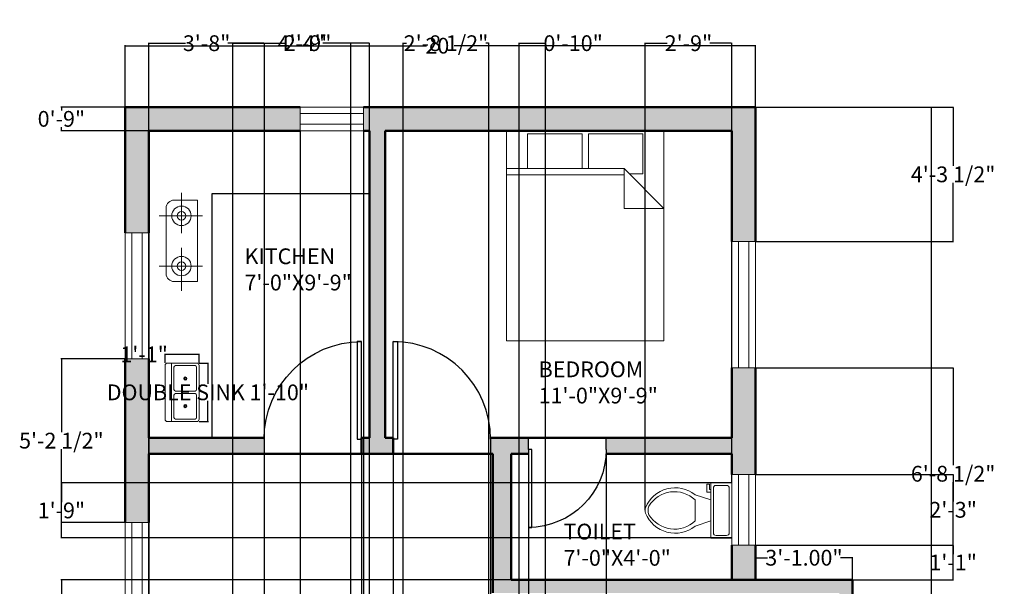
# Model space of a CAD drawing. Units: inches. Extents: x -19 to 356, y -14 to 509.
# Tile 3 of 3: x -19 to 356, y 293 to 509. Entities that reach past the tile are written whole.
import ezdxf

# ---------------------------------------------------------------- set-up
doc = ezdxf.new("R2010")
doc.units = ezdxf.units.IN
doc.header["$MEASUREMENT"] = 0
for name, color, linetype, lineweight in [('A-ANNO-DIMS', 7, 'Continuous', 18), ('A-ANNO-TEXT', 7, 'Continuous', 18), ('A-AREA-IDEN', 7, 'Continuous', 25), ('A-DOOR', 3, 'Continuous', 25), ('A-EQPM', 7, 'Continuous', 18), ('A-FLOR-CASE', 8, 'Continuous', 25), ('A-FLOR-FIXT', 9, 'Continuous', 18), ('A-FURN', 8, 'Continuous', 18), ('A-GLAZ', 5, 'Continuous', 18), ('A-WALL', 7, 'Continuous', 50), ('A-WALL-PATT', 4, 'Continuous', 13)]:
    doc.layers.add(name, color=color, linetype=linetype, lineweight=lineweight)
doc.styles.get("Standard").update_dxf_attribs({"font": 'arial.ttf'})
doc.dimstyles.get("Standard").update_dxf_attribs({"dimtxt": 6, "dimasz": 0.18, "dimexe": 0.18, "dimexo": 0.0625, "dimgap": 0.09, "dimtad": 0, "dimtih": 1, "dimtoh": 1, "dimzin": 0, "dimdsep": 46, "dimlunit": 3, "dimtxsty": 'Standard', "dimcen": 0.09, "dimadec": 0, "dimazin": 0, "dimtfac": 1, "dimtofl": 0, "dimtmove": 0, "dimatfit": 3, "dimfxl": 1, "dimtolj": 1, "dimtzin": 0, "dimarcsym": 0})

# ---------------------------------------------------------------- blocks, each defined once
blk = doc.blocks.new('*U2')
for p, q in [((0, 0), (0, -6)), ((40, 0), (40, -6))]:
    blk.add_line(p, q)
blk.add_lwpolyline([(0, 0), (0, 40), (1.75, 40), (1.75, 0)], close=True)
blk.add_arc((0, 0), 40, 0, 90)
blk = doc.blocks.new('*U4')
for p, q in [((9.5, -6), (9.5, -2)), ((-10, -8.5), (-8, -8.5)), ((-10, -9.5), (-10, -8.5)), ((-7, -9.5), (-10, -9.5)), ((-8, -8.5), (-8, -8)), ((-7, -8), (-7, -9.5)), ((-4, -8), (-6, -14)), ((4, -8), (6, -14)), ((4, -14), (-4, -14))]:
    blk.add_line(p, q)
blk.add_lwpolyline([(10.5, -8), (10.5, 0), (-10.5, 0), (-10.5, -8)], close=True)
for points in [[(-9.5, -2), (-9.5, -6)], [(8.5, -1), (-8.5, -1)], [(-8.5, -7), (8.5, -7)]]:
    blk.add_lwpolyline(points)
for centre, radius, start, end in [((-8.62, -1.88), 0.884, 81.8699, 188.1301), ((8.62, -1.88), 0.884, 351.8699, 98.1301), ((-8.62, -6.12), 0.884, 171.8699, 278.1301), ((8.62, -6.12), 0.884, 261.8699, 8.1301), ((3.52, -21.58), 12.17, 141.4691, 247.9714), ((4.2, -21.82), 11.33, 136.3677, 238.9468), ((-3.52, -21.58), 12.17, 292.0284, 38.5307), ((-4.2, -21.82), 11.33, 301.053, 43.6321), ((0, -27.88), 4, 245.7318, 294.2682), ((0, -29), 4, 254.8605, 285.1395)]:
    blk.add_arc(centre, radius, start, end)
blk = doc.blocks.new('Bed - Queen')
for p, q in [((0, -80.00003), (0, 0)), ((0, 0), (59.99999, 0)), ((59.99999, 0), (59.99999, -80.00003)), ((7.99999, -1.2), (28.79998, -1.2)), ((7.99999, -14.4), (7.99999, -1.2)), ((28.79998, -1.2), (28.79998, -14.4)), ((31.19999, -1.2), (51.99999, -1.2)), ((31.19999, -14.4), (31.19999, -1.2)), ((51.99999, -1.2), (51.99999, -16.4)), ((0, -14.4), (44.8, -14.4)), ((59.99999, -29.6), (44.8, -14.4)), ((44.8, -14.4), (44.8, -29.6)), ((44.8, -16.8), (0, -16.8)), ((51.99999, -16.4), (46.79936, -16.4)), ((44.8, -29.6), (59.99999, -29.6)), ((59.99999, -80.00003), (0, -80.00003))]:
    blk.add_line(p, q)
blk = doc.blocks.new('Sink-double - 36 in top')
for p, q in [((-18, -4), (18, -4)), ((-0.75, -18.5), (-0.75, -6.5)), ((0.75, -6.5), (0.75, -18.5))]:
    blk.add_line(p, q)
for points in [[(-16.5, 0), (16.5, 0)], [(-18, -19.5), (-18, -1.5)], [(-15.5, -5.5), (-1.75, -5.5)], [(1.75, -5.5), (15.5, -5.5)], [(18, -1.5), (18, -19.5)], [(-16.5, -18.5), (-16.5, -6.5)], [(16.5, -6.5), (16.5, -18.5)], [(16.5, -21), (-16.5, -21)], [(-1.75, -19.5), (-15.5, -19.5)], [(15.5, -19.5), (1.75, -19.5)]]:
    blk.add_lwpolyline(points)
for centre, radius in [((-8.5, -12.5), 1), ((-8.5, -12.5), 0.5), ((8.5, -12.5), 1), ((8.5, -12.5), 0.5)]:
    blk.add_circle(centre, radius)
for centre, radius, start, end in [((-16.5, -1.5), 1.5, 90, 180), ((16.5, -1.5), 1.5, 0, 90), ((-15.5, -6.5), 1, 90, 180), ((-1.75, -6.5), 1, 0, 90), ((1.75, -6.5), 1, 90, 180), ((15.5, -6.5), 1, 0, 90), ((-16.5, -19.5), 1.5, 180, 270), ((-15.5, -18.5), 1, 180, 270), ((-1.75, -18.5), 1, 270, 0), ((1.75, -18.5), 1, 180, 270), ((15.5, -18.5), 1, 270, 0), ((16.5, -19.5), 1.5, 270, 0)]:
    blk.add_arc(centre, radius, start, end)
blk = doc.blocks.new('*D7')
at = {"layer": 'A-ANNO-DIMS', "color": 0, "lineweight": -2, "transparency": 16777216}
for p, q in [((21.6, 475.44), (21.6, 498.91)), ((261.6, 475.44), (261.6, 498.91)), ((21.78, 498.73), (136.37, 498.73)), ((261.42, 498.73), (146.83, 498.73))]:
    blk.add_line(p, q, dxfattribs=at)
at = {"layer": 'A-ANNO-DIMS', "color": 0, "transparency": 16777216}
for points in [[(21.78, 498.76), (21.78, 498.7), (21.6, 498.73)], [(261.42, 498.76), (261.42, 498.7), (261.6, 498.73)]]:
    blk.add_solid(points, dxfattribs=at)
at = {"layer": 'Defpoints', "color": 0, "transparency": 16777216}
for p in [(261.6, 498.73), (21.6, 475.37), (261.6, 475.37)]:
    blk.add_point(p, dxfattribs=at)
at = {"layer": 'A-ANNO-DIMS', "color": 0, "transparency": 16777216, "insert": (141.6, 498.73), "char_height": 6, "attachment_point": 5}
blk.add_mtext("\\A1;20'", dxfattribs=at)
blk = doc.blocks.new('*D8')
at = {"layer": 'A-ANNO-DIMS', "color": 0, "lineweight": -2, "transparency": 16777216}
for p, q in [((261.66, 475.37), (328.76, 475.37)), ((328.58, 475.19), (328.58, 250.53)), ((328.58, 19.55), (328.58, 244.22)), ((261.66, 19.37), (328.76, 19.37))]:
    blk.add_line(p, q, dxfattribs=at)
at = {"layer": 'A-ANNO-DIMS', "color": 0, "transparency": 16777216}
for points in [[(328.55, 475.19), (328.61, 475.19), (328.58, 475.37)], [(328.55, 19.55), (328.61, 19.55), (328.58, 19.37)]]:
    blk.add_solid(points, dxfattribs=at)
at = {"layer": 'Defpoints', "color": 0, "transparency": 16777216}
for p in [(261.6, 475.37), (328.58, 475.37), (261.6, 19.37)]:
    blk.add_point(p, dxfattribs=at)
at = {"layer": 'A-ANNO-DIMS', "color": 0, "transparency": 16777216, "insert": (328.58, 247.37), "char_height": 6, "attachment_point": 5}
blk.add_mtext("\\A1;38'", dxfattribs=at)
blk = doc.blocks.new('*D9')
at = {"layer": 'A-ANNO-DIMS', "color": 0, "lineweight": -2, "transparency": 16777216}
for p, q in [((261.6, 295.44), (261.6, 303.93)), ((261.78, 303.75), (266.21, 303.75)), ((298.42, 303.75), (293.99, 303.75)), ((298.6, 295.44), (298.6, 303.93))]:
    blk.add_line(p, q, dxfattribs=at)
at = {"layer": 'A-ANNO-DIMS', "color": 0, "transparency": 16777216}
for points in [[(261.78, 303.78), (261.78, 303.72), (261.6, 303.75)], [(298.42, 303.78), (298.42, 303.72), (298.6, 303.75)]]:
    blk.add_solid(points, dxfattribs=at)
at = {"layer": 'Defpoints', "color": 0, "transparency": 16777216}
for p in [(298.6, 303.75), (261.6, 295.37), (298.6, 295.37)]:
    blk.add_point(p, dxfattribs=at)
at = {"layer": 'A-ANNO-DIMS', "color": 0, "transparency": 16777216, "insert": (280.1, 303.75), "char_height": 6, "attachment_point": 5}
blk.add_mtext('\\A1;3\'-1.00"', dxfattribs=at)
blk = doc.blocks.new('GLAZ-UNIT-48IN')
for p, q in [((0, 48), (0, 0)), ((4, 48), (4, 0))]:
    blk.add_line(p, q)
blk = doc.blocks.new('*D17')
at = {"layer": 'A-ANNO-DIMS', "color": 0, "lineweight": -2, "transparency": 16777216}
for p, q in [((49.79, 377.86), (53.25, 377.86)), ((53.07, 377.68), (53.07, 369.93)), ((53.07, 355.79), (53.07, 363.54)), ((49.79, 355.61), (53.25, 355.61))]:
    blk.add_line(p, q, dxfattribs=at)
at = {"layer": 'A-ANNO-DIMS', "color": 0, "transparency": 16777216}
for points in [[(53.04, 377.68), (53.1, 377.68), (53.07, 377.86)], [(53.04, 355.79), (53.1, 355.79), (53.07, 355.61)]]:
    blk.add_solid(points, dxfattribs=at)
at = {"layer": 'Defpoints', "color": 0, "transparency": 16777216}
for p in [(49.73, 377.86), (53.07, 377.86), (49.73, 355.61)]:
    blk.add_point(p, dxfattribs=at)
at = {"layer": 'A-ANNO-DIMS', "color": 0, "transparency": 16777216, "insert": (53.07, 366.73), "char_height": 6, "attachment_point": 5}
blk.add_mtext('\\A1;DOUBLE SINK 1\'-10"', dxfattribs=at)
blk = doc.blocks.new('*D18')
at = {"layer": 'A-ANNO-DIMS', "color": 0, "lineweight": -2, "transparency": 16777216}
for p, q in [((36.75, 381.19), (36.57, 381.19)), ((36.75, 377.92), (36.75, 381.37)), ((49.55, 381.19), (36.93, 381.19)), ((49.73, 377.92), (49.73, 381.37))]:
    blk.add_line(p, q, dxfattribs=at)
at = {"layer": 'A-ANNO-DIMS', "color": 0, "transparency": 16777216}
for points in [[(36.93, 381.22), (36.93, 381.16), (36.75, 381.19)], [(49.55, 381.22), (49.55, 381.16), (49.73, 381.19)]]:
    blk.add_solid(points, dxfattribs=at)
at = {"layer": 'Defpoints', "color": 0, "transparency": 16777216}
for p in [(36.75, 381.19), (36.75, 377.86), (49.73, 377.86)]:
    blk.add_point(p, dxfattribs=at)
at = {"layer": 'A-ANNO-DIMS', "color": 0, "transparency": 16777216, "insert": (28.79, 381.19), "char_height": 6, "attachment_point": 5}
blk.add_mtext('\\A1;1\'-1"', dxfattribs=at)
blk = doc.blocks.new('*D21')
at = {"layer": 'A-ANNO-DIMS', "color": 0, "lineweight": -2, "transparency": 16777216}
for p, q in [((30.6, 48.44), (30.6, 499.87)), ((30.78, 499.69), (44.54, 499.69)), ((74.42, 499.69), (60.66, 499.69)), ((74.6, 39.44), (74.6, 499.87))]:
    blk.add_line(p, q, dxfattribs=at)
at = {"layer": 'A-ANNO-DIMS', "color": 0, "transparency": 16777216}
for points in [[(30.78, 499.72), (30.78, 499.66), (30.6, 499.69)], [(74.42, 499.72), (74.42, 499.66), (74.6, 499.69)]]:
    blk.add_solid(points, dxfattribs=at)
at = {"layer": 'Defpoints', "color": 0, "transparency": 16777216}
for p in [(74.6, 499.69), (30.6, 48.37), (74.6, 39.37)]:
    blk.add_point(p, dxfattribs=at)
at = {"layer": 'A-ANNO-DIMS', "color": 0, "transparency": 16777216, "insert": (52.6, 499.69), "char_height": 6, "attachment_point": 5}
blk.add_mtext('\\A1;3\'-8"', dxfattribs=at)
blk = doc.blocks.new('*D22')
at = {"layer": 'A-ANNO-DIMS', "color": 0, "lineweight": -2, "transparency": 16777216}
for p, q in [((74.6, 39.44), (74.6, 499.87)), ((74.78, 499.69), (82.95, 499.69)), ((107.35, 499.69), (99.18, 499.69)), ((107.53, 39.44), (107.53, 499.87))]:
    blk.add_line(p, q, dxfattribs=at)
at = {"layer": 'A-ANNO-DIMS', "color": 0, "transparency": 16777216}
for points in [[(74.78, 499.72), (74.78, 499.66), (74.6, 499.69)], [(107.35, 499.72), (107.35, 499.66), (107.53, 499.69)]]:
    blk.add_solid(points, dxfattribs=at)
at = {"layer": 'Defpoints', "color": 0, "transparency": 16777216}
for p in [(107.53, 499.69), (74.6, 39.37), (107.53, 39.37)]:
    blk.add_point(p, dxfattribs=at)
at = {"layer": 'A-ANNO-DIMS', "color": 0, "transparency": 16777216, "insert": (91.07, 499.69), "char_height": 6, "attachment_point": 5}
blk.add_mtext('\\A1;2\'-9"', dxfattribs=at)
blk = doc.blocks.new('*D23')
at = {"layer": 'A-ANNO-DIMS', "color": 0, "lineweight": -2, "transparency": 16777216}
for p, q in [((30.6, 466.31), (30.6, -5.12)), ((88.28, 466.31), (88.28, -5.12)), ((30.78, -4.94), (44.27, -4.94)), ((88.1, -4.94), (74.62, -4.94))]:
    blk.add_line(p, q, dxfattribs=at)
at = {"layer": 'A-ANNO-DIMS', "color": 0, "transparency": 16777216}
for points in [[(30.78, -4.91), (30.78, -4.97), (30.6, -4.94)], [(88.1, -4.91), (88.1, -4.97), (88.28, -4.94)]]:
    blk.add_solid(points, dxfattribs=at)
at = {"layer": 'Defpoints', "color": 0, "transparency": 16777216}
for p in [(30.6, 466.37), (88.28, 466.37), (88.28, -4.94)]:
    blk.add_point(p, dxfattribs=at)
at = {"layer": 'A-ANNO-DIMS', "color": 0, "transparency": 16777216, "insert": (59.44, -4.94), "char_height": 6, "attachment_point": 5}
blk.add_mtext('\\A1;4\'-9 1/2"', dxfattribs=at)
blk = doc.blocks.new('*D24')
at = {"layer": 'A-ANNO-DIMS', "color": 0, "lineweight": -2, "transparency": 16777216}
for p, q in [((88.28, 466.31), (88.28, -5.12)), ((112.28, 466.31), (112.28, -5.12)), ((88.46, -4.94), (92.17, -4.94)), ((112.1, -4.94), (108.4, -4.94))]:
    blk.add_line(p, q, dxfattribs=at)
at = {"layer": 'A-ANNO-DIMS', "color": 0, "transparency": 16777216}
for points in [[(88.46, -4.91), (88.46, -4.97), (88.28, -4.94)], [(112.1, -4.91), (112.1, -4.97), (112.28, -4.94)]]:
    blk.add_solid(points, dxfattribs=at)
at = {"layer": 'Defpoints', "color": 0, "transparency": 16777216}
for p in [(88.28, 466.37), (112.28, 466.37), (112.28, -4.94)]:
    blk.add_point(p, dxfattribs=at)
at = {"layer": 'A-ANNO-DIMS', "color": 0, "transparency": 16777216, "insert": (100.28, -4.94), "char_height": 6, "attachment_point": 5}
blk.add_mtext('\\A1;2\'-0"', dxfattribs=at)
blk = doc.blocks.new('*D28')
at = {"layer": 'A-ANNO-DIMS', "color": 0, "lineweight": -2, "transparency": 16777216}
for p, q in [((21.54, 379.49), (-2.9, 379.49)), ((-2.72, 379.31), (-2.72, 351.53)), ((-2.72, 317.37), (-2.72, 345.15)), ((21.54, 317.19), (-2.9, 317.19))]:
    blk.add_line(p, q, dxfattribs=at)
at = {"layer": 'A-ANNO-DIMS', "color": 0, "transparency": 16777216}
for points in [[(-2.75, 379.31), (-2.69, 379.31), (-2.72, 379.49)], [(-2.75, 317.37), (-2.69, 317.37), (-2.72, 317.19)]]:
    blk.add_solid(points, dxfattribs=at)
at = {"layer": 'Defpoints', "color": 0, "transparency": 16777216}
for p in [(-2.72, 379.49), (21.6, 379.49), (21.6, 317.19)]:
    blk.add_point(p, dxfattribs=at)
at = {"layer": 'A-ANNO-DIMS', "color": 0, "transparency": 16777216, "insert": (-2.72, 348.34), "char_height": 6, "attachment_point": 5}
blk.add_mtext('\\A1;5\'-2 1/2"', dxfattribs=at)
blk = doc.blocks.new('*D30')
at = {"layer": 'A-ANNO-DIMS', "color": 0, "lineweight": -2, "transparency": 16777216}
for p, q in [((74.5, 343.31), (74.5, -5.12)), ((111.6, 343.31), (111.6, -5.12)), ((74.68, -4.94), (84.99, -4.94)), ((111.42, -4.94), (101.11, -4.94))]:
    blk.add_line(p, q, dxfattribs=at)
at = {"layer": 'A-ANNO-DIMS', "color": 0, "transparency": 16777216}
for points in [[(74.68, -4.91), (74.68, -4.97), (74.5, -4.94)], [(111.42, -4.91), (111.42, -4.97), (111.6, -4.94)]]:
    blk.add_solid(points, dxfattribs=at)
at = {"layer": 'Defpoints', "color": 0, "transparency": 16777216}
for p in [(74.5, 343.37), (111.6, 343.37), (111.6, -4.94)]:
    blk.add_point(p, dxfattribs=at)
at = {"layer": 'A-ANNO-DIMS', "color": 0, "transparency": 16777216, "insert": (93.05, -4.94), "char_height": 6, "attachment_point": 5}
blk.add_mtext('\\A1;3\'-1"', dxfattribs=at)
blk = doc.blocks.new('*D31')
at = {"layer": 'A-ANNO-DIMS', "color": 0, "lineweight": -2, "transparency": 16777216}
for p, q in [((123.6, 343.31), (123.6, -5.12)), ((160.72, 343.31), (160.72, -5.12)), ((123.78, -4.94), (134.1, -4.94)), ((160.54, -4.94), (150.22, -4.94))]:
    blk.add_line(p, q, dxfattribs=at)
at = {"layer": 'A-ANNO-DIMS', "color": 0, "transparency": 16777216}
for points in [[(123.78, -4.91), (123.78, -4.97), (123.6, -4.94)], [(160.54, -4.91), (160.54, -4.97), (160.72, -4.94)]]:
    blk.add_solid(points, dxfattribs=at)
at = {"layer": 'Defpoints', "color": 0, "transparency": 16777216}
for p in [(123.6, 343.37), (160.72, 343.37), (160.72, -4.94)]:
    blk.add_point(p, dxfattribs=at)
at = {"layer": 'A-ANNO-DIMS', "color": 0, "transparency": 16777216, "insert": (142.16, -4.94), "char_height": 6, "attachment_point": 5}
blk.add_mtext('\\A1;3\'-1"', dxfattribs=at)
blk = doc.blocks.new('*D32')
at = {"layer": 'A-ANNO-DIMS', "color": 0, "lineweight": -2, "transparency": 16777216}
for p, q in [((127.47, 153.44), (127.47, 499.87)), ((127.65, 499.69), (128.66, 499.69)), ((159.89, 499.69), (158.88, 499.69)), ((160.07, 153.44), (160.07, 499.87))]:
    blk.add_line(p, q, dxfattribs=at)
at = {"layer": 'A-ANNO-DIMS', "color": 0, "transparency": 16777216}
for points in [[(127.65, 499.72), (127.65, 499.66), (127.47, 499.69)], [(159.89, 499.72), (159.89, 499.66), (160.07, 499.69)]]:
    blk.add_solid(points, dxfattribs=at)
at = {"layer": 'Defpoints', "color": 0, "transparency": 16777216}
for p in [(160.07, 499.69), (127.47, 153.37), (160.07, 153.37)]:
    blk.add_point(p, dxfattribs=at)
at = {"layer": 'A-ANNO-DIMS', "color": 0, "transparency": 16777216, "insert": (143.77, 499.69), "char_height": 6, "attachment_point": 5}
blk.add_mtext('\\A1;2\'-8 1/2"', dxfattribs=at)
blk = doc.blocks.new('*D33')
at = {"layer": 'A-ANNO-DIMS', "color": 0, "lineweight": -2, "transparency": 16777216}
for p, q in [((74.6, 153.44), (74.6, 499.87)), ((74.78, 499.69), (82.95, 499.69)), ((107.35, 499.69), (99.18, 499.69)), ((107.53, 153.44), (107.53, 499.87))]:
    blk.add_line(p, q, dxfattribs=at)
at = {"layer": 'A-ANNO-DIMS', "color": 0, "transparency": 16777216}
for points in [[(74.78, 499.72), (74.78, 499.66), (74.6, 499.69)], [(107.35, 499.72), (107.35, 499.66), (107.53, 499.69)]]:
    blk.add_solid(points, dxfattribs=at)
at = {"layer": 'Defpoints', "color": 0, "transparency": 16777216}
for p in [(107.53, 499.69), (74.6, 153.37), (107.53, 153.37)]:
    blk.add_point(p, dxfattribs=at)
at = {"layer": 'A-ANNO-DIMS', "color": 0, "transparency": 16777216, "insert": (91.07, 499.69), "char_height": 6, "attachment_point": 5}
blk.add_mtext('\\A1;2\'-9"', dxfattribs=at)
blk = doc.blocks.new('*D34')
at = {"layer": 'A-ANNO-DIMS', "color": 0, "lineweight": -2, "transparency": 16777216}
for p, q in [((175.13, 343.31), (175.13, -5.12)), ((204.73, 343.31), (204.73, -5.12)), ((175.31, -4.94), (204.55, -4.94)), ((204.73, -4.94), (204.91, -4.94))]:
    blk.add_line(p, q, dxfattribs=at)
at = {"layer": 'A-ANNO-DIMS', "color": 0, "transparency": 16777216}
for points in [[(175.31, -4.91), (175.31, -4.97), (175.13, -4.94)], [(204.55, -4.91), (204.55, -4.97), (204.73, -4.94)]]:
    blk.add_solid(points, dxfattribs=at)
at = {"layer": 'Defpoints', "color": 0, "transparency": 16777216}
for p in [(175.13, 343.37), (204.73, 343.37), (204.73, -4.94)]:
    blk.add_point(p, dxfattribs=at)
at = {"layer": 'A-ANNO-DIMS', "color": 0, "transparency": 16777216, "insert": (220.01, -4.94), "char_height": 6, "attachment_point": 5}
blk.add_mtext('\\A1;2\'-5 1/2"', dxfattribs=at)
blk = doc.blocks.new('*D36')
at = {"layer": 'A-ANNO-DIMS', "color": 0, "lineweight": -2, "transparency": 16777216}
for p, q in [((261.66, 475.37), (337.09, 475.37)), ((336.91, 475.19), (336.91, 452.94)), ((336.91, 424.29), (336.91, 446.55)), ((261.66, 424.11), (337.09, 424.11))]:
    blk.add_line(p, q, dxfattribs=at)
at = {"layer": 'A-ANNO-DIMS', "color": 0, "transparency": 16777216}
for points in [[(336.88, 475.19), (336.94, 475.19), (336.91, 475.37)], [(336.88, 424.29), (336.94, 424.29), (336.91, 424.11)]]:
    blk.add_solid(points, dxfattribs=at)
at = {"layer": 'Defpoints', "color": 0, "transparency": 16777216}
for p in [(261.6, 475.37), (336.91, 475.37), (261.6, 424.11)]:
    blk.add_point(p, dxfattribs=at)
at = {"layer": 'A-ANNO-DIMS', "color": 0, "transparency": 16777216, "insert": (336.91, 449.74), "char_height": 6, "attachment_point": 5}
blk.add_mtext('\\A1;4\'-3 1/2"', dxfattribs=at)
blk = doc.blocks.new('*D37')
at = {"layer": 'A-ANNO-DIMS', "color": 0, "lineweight": -2, "transparency": 16777216}
for p, q in [((261.66, 376.11), (337.09, 376.11)), ((336.91, 375.93), (336.91, 338.94)), ((336.91, 295.55), (336.91, 332.55)), ((261.66, 295.37), (337.09, 295.37))]:
    blk.add_line(p, q, dxfattribs=at)
at = {"layer": 'A-ANNO-DIMS', "color": 0, "transparency": 16777216}
for points in [[(336.88, 375.93), (336.94, 375.93), (336.91, 376.11)], [(336.88, 295.55), (336.94, 295.55), (336.91, 295.37)]]:
    blk.add_solid(points, dxfattribs=at)
at = {"layer": 'Defpoints', "color": 0, "transparency": 16777216}
for p in [(261.6, 376.11), (336.91, 376.11), (261.6, 295.37)]:
    blk.add_point(p, dxfattribs=at)
at = {"layer": 'A-ANNO-DIMS', "color": 0, "transparency": 16777216, "insert": (336.91, 335.74), "char_height": 6, "attachment_point": 5}
blk.add_mtext('\\A1;6\'-8 1/2"', dxfattribs=at)
blk = doc.blocks.new('*D38')
at = {"layer": 'A-ANNO-DIMS', "color": 0, "lineweight": -2, "transparency": 16777216}
for p, q in [((261.66, 335.44), (337.09, 335.44)), ((336.91, 335.26), (336.91, 325.16)), ((336.91, 308.75), (336.91, 318.85)), ((261.66, 308.57), (337.09, 308.57))]:
    blk.add_line(p, q, dxfattribs=at)
at = {"layer": 'A-ANNO-DIMS', "color": 0, "transparency": 16777216}
for points in [[(336.88, 335.26), (336.94, 335.26), (336.91, 335.44)], [(336.88, 308.75), (336.94, 308.75), (336.91, 308.57)]]:
    blk.add_solid(points, dxfattribs=at)
at = {"layer": 'Defpoints', "color": 0, "transparency": 16777216}
for p in [(261.6, 335.44), (336.91, 335.44), (261.6, 308.57)]:
    blk.add_point(p, dxfattribs=at)
at = {"layer": 'A-ANNO-DIMS', "color": 0, "transparency": 16777216, "insert": (336.91, 322), "char_height": 6, "attachment_point": 5}
blk.add_mtext('\\A1;2\'-3"', dxfattribs=at)
blk = doc.blocks.new('*D39')
at = {"layer": 'A-ANNO-DIMS', "color": 0, "lineweight": -2, "transparency": 16777216}
for p, q in [((261.66, 308.57), (337.09, 308.57)), ((336.91, 308.39), (336.91, 305.07)), ((336.91, 295.55), (336.91, 298.87)), ((261.66, 295.37), (337.09, 295.37))]:
    blk.add_line(p, q, dxfattribs=at)
at = {"layer": 'A-ANNO-DIMS', "color": 0, "transparency": 16777216}
for points in [[(336.88, 308.39), (336.94, 308.39), (336.91, 308.57)], [(336.88, 295.55), (336.94, 295.55), (336.91, 295.37)]]:
    blk.add_solid(points, dxfattribs=at)
at = {"layer": 'Defpoints', "color": 0, "transparency": 16777216}
for p in [(261.6, 308.57), (336.91, 308.57), (261.6, 295.37)]:
    blk.add_point(p, dxfattribs=at)
at = {"layer": 'A-ANNO-DIMS', "color": 0, "transparency": 16777216, "insert": (336.91, 301.97), "char_height": 6, "attachment_point": 5}
blk.add_mtext('\\A1;1\'-1"', dxfattribs=at)
blk = doc.blocks.new('*D40')
at = {"layer": 'A-ANNO-DIMS', "color": 0, "lineweight": -2, "transparency": 16777216}
for p, q in [((168.54, 295.37), (-2.9, 295.37)), ((-2.72, 295.19), (-2.72, 251.53)), ((-2.72, 201.55), (-2.72, 245.22)), ((161.54, 201.37), (-2.9, 201.37))]:
    blk.add_line(p, q, dxfattribs=at)
at = {"layer": 'A-ANNO-DIMS', "color": 0, "transparency": 16777216}
for points in [[(-2.75, 295.19), (-2.69, 295.19), (-2.72, 295.37)], [(-2.75, 201.55), (-2.69, 201.55), (-2.72, 201.37)]]:
    blk.add_solid(points, dxfattribs=at)
at = {"layer": 'Defpoints', "color": 0, "transparency": 16777216}
for p in [(-2.72, 295.37), (168.6, 295.37), (161.6, 201.37)]:
    blk.add_point(p, dxfattribs=at)
at = {"layer": 'A-ANNO-DIMS', "color": 0, "transparency": 16777216, "insert": (-2.72, 248.37), "char_height": 6, "attachment_point": 5}
blk.add_mtext('\\A1;7\'-10"', dxfattribs=at)
blk = doc.blocks.new('*D44')
at = {"layer": 'A-ANNO-DIMS', "color": 0, "lineweight": -2, "transparency": 16777216}
for p, q in [((62.64, 21.44), (62.64, 499.87)), ((62.82, 499.69), (80.44, 499.69)), ((114.42, 499.69), (96.81, 499.69)), ((114.6, 21.44), (114.6, 499.87))]:
    blk.add_line(p, q, dxfattribs=at)
at = {"layer": 'A-ANNO-DIMS', "color": 0, "transparency": 16777216}
for points in [[(62.82, 499.72), (62.82, 499.66), (62.64, 499.69)], [(114.42, 499.72), (114.42, 499.66), (114.6, 499.69)]]:
    blk.add_solid(points, dxfattribs=at)
at = {"layer": 'Defpoints', "color": 0, "transparency": 16777216}
for p in [(114.6, 499.69), (62.64, 21.37), (114.6, 21.37)]:
    blk.add_point(p, dxfattribs=at)
at = {"layer": 'A-ANNO-DIMS', "color": 0, "transparency": 16777216, "insert": (88.62, 499.69), "char_height": 6, "attachment_point": 5}
blk.add_mtext('\\A1;4\'-4"', dxfattribs=at)
blk = doc.blocks.new('*D45')
at = {"layer": 'A-ANNO-DIMS', "color": 0, "lineweight": -2, "transparency": 16777216}
for p, q in [((21.54, 475.37), (-2.9, 475.37)), ((-2.72, 475.19), (-2.72, 474.03)), ((30.54, 466.37), (-2.9, 466.37)), ((-2.72, 466.55), (-2.72, 467.72))]:
    blk.add_line(p, q, dxfattribs=at)
at = {"layer": 'A-ANNO-DIMS', "color": 0, "transparency": 16777216}
for points in [[(-2.75, 475.19), (-2.69, 475.19), (-2.72, 475.37)], [(-2.75, 466.55), (-2.69, 466.55), (-2.72, 466.37)]]:
    blk.add_solid(points, dxfattribs=at)
at = {"layer": 'Defpoints', "color": 0, "transparency": 16777216}
for p in [(21.6, 475.37), (-2.72, 466.37), (30.6, 466.37)]:
    blk.add_point(p, dxfattribs=at)
at = {"layer": 'A-ANNO-DIMS', "color": 0, "transparency": 16777216, "insert": (-2.72, 470.87), "char_height": 6, "attachment_point": 5}
blk.add_mtext('\\A1;0\'-9"', dxfattribs=at)
blk = doc.blocks.new('*D47')
at = {"layer": 'A-ANNO-DIMS', "color": 0, "lineweight": -2, "transparency": 16777216}
for p, q in [((171.6, 206.44), (171.6, 499.87)), ((171.78, 499.69), (181.42, 499.69)), ((181.6, 206.44), (181.6, 499.87)), ((181.6, 499.69), (181.78, 499.69))]:
    blk.add_line(p, q, dxfattribs=at)
at = {"layer": 'A-ANNO-DIMS', "color": 0, "transparency": 16777216}
for points in [[(171.78, 499.72), (171.78, 499.66), (171.6, 499.69)], [(181.42, 499.72), (181.42, 499.66), (181.6, 499.69)]]:
    blk.add_solid(points, dxfattribs=at)
at = {"layer": 'Defpoints', "color": 0, "transparency": 16777216}
for p in [(181.6, 499.69), (171.6, 206.37), (181.6, 206.37)]:
    blk.add_point(p, dxfattribs=at)
at = {"layer": 'A-ANNO-DIMS', "color": 0, "transparency": 16777216, "insert": (192.18, 499.69), "char_height": 6, "attachment_point": 5}
blk.add_mtext('\\A1;0\'-10"', dxfattribs=at)
blk = doc.blocks.new('*D49')
at = {"layer": 'A-ANNO-DIMS', "color": 0, "lineweight": -2, "transparency": 16777216}
for p, q in [((219.6, 321.83), (219.6, 499.87)), ((219.78, 499.69), (227.98, 499.69)), ((252.42, 499.69), (244.22, 499.69)), ((252.6, 332.33), (252.6, 499.87))]:
    blk.add_line(p, q, dxfattribs=at)
at = {"layer": 'A-ANNO-DIMS', "color": 0, "transparency": 16777216}
for points in [[(219.78, 499.72), (219.78, 499.66), (219.6, 499.69)], [(252.42, 499.72), (252.42, 499.66), (252.6, 499.69)]]:
    blk.add_solid(points, dxfattribs=at)
at = {"layer": 'Defpoints', "color": 0, "transparency": 16777216}
for p in [(252.6, 499.69), (252.6, 332.27), (219.6, 321.77)]:
    blk.add_point(p, dxfattribs=at)
at = {"layer": 'A-ANNO-DIMS', "color": 0, "transparency": 16777216, "insert": (236.1, 499.69), "char_height": 6, "attachment_point": 5}
blk.add_mtext('\\A1;2\'-9"', dxfattribs=at)
blk = doc.blocks.new('*D50')
at = {"layer": 'A-ANNO-DIMS', "color": 0, "lineweight": -2, "transparency": 16777216}
for p, q in [((252.54, 332.27), (-2.9, 332.27)), ((-2.72, 332.09), (-2.72, 324.92)), ((-2.72, 311.45), (-2.72, 318.61)), ((252.54, 311.27), (-2.9, 311.27))]:
    blk.add_line(p, q, dxfattribs=at)
at = {"layer": 'A-ANNO-DIMS', "color": 0, "transparency": 16777216}
for points in [[(-2.75, 332.09), (-2.69, 332.09), (-2.72, 332.27)], [(-2.75, 311.45), (-2.69, 311.45), (-2.72, 311.27)]]:
    blk.add_solid(points, dxfattribs=at)
at = {"layer": 'Defpoints', "color": 0, "transparency": 16777216}
for p in [(-2.72, 332.27), (252.6, 332.27), (252.6, 311.27)]:
    blk.add_point(p, dxfattribs=at)
at = {"layer": 'A-ANNO-DIMS', "color": 0, "transparency": 16777216, "insert": (-2.72, 321.77), "char_height": 6, "attachment_point": 5}
blk.add_mtext('\\A1;1\'-9"', dxfattribs=at)

msp = doc.modelspace()

# ---------------------------------------------------------------- hatches: boundary and pattern name
at = {"layer": 'A-WALL-PATT'}
h = msp.add_hatch(color=256, dxfattribs=at)
h.dxf.hatch_style = 1
h.paths.add_polyline_path([(30.6, 466.373), (88.282, 466.373), (88.282, 475.373), (21.6, 475.373), (21.6, 427.492), (30.6, 427.492)])
h.paths.add_polyline_path([(261.6, 475.373), (112.282, 475.373), (112.282, 466.373), (114.6, 466.373), (114.6, 349.373), (111.606, 349.373), (111.606, 348.938), (111.606, 343.373), (123.6, 343.373), (123.6, 349.373), (120.6, 349.373), (120.6, 466.373), (252.6, 466.373), (252.6, 424.113), (261.6, 424.113)])
h.paths.add_polyline_path([(261.6, 376.113), (252.6, 376.113), (252.6, 349.373), (204.767, 349.373), (204.767, 344.927, -0.0131156), (204.727, 343.373), (252.6, 343.373), (252.6, 335.439), (261.6, 335.439)])
h.paths.add_polyline_path([(261.6, 308.567), (252.6, 308.567), (252.6, 295.373), (261.6, 295.373)], flags=17)
h.paths.add_polyline_path([(298.6, 295.373), (168.6, 295.373), (168.6, 343.373), (175.128, 343.373), (175.128, 344.927), (175.128, 349.373), (160.722, 349.373, -0.0029301), (160.724, 348.938), (160.724, 343.373), (161.6, 343.373), (161.6, 290.373), (293.6, 290.373), (293.6, 281.12), (298.6, 281.12)])
h = msp.add_hatch(color=256, dxfattribs=at)
h.dxf.hatch_style = 1
h.paths.add_polyline_path([(74.504, 349.373), (30.6, 349.373), (30.6, 379.492), (21.6, 379.492), (21.6, 317.187), (30.6, 317.187), (30.6, 343.373), (74.504, 343.373)])
h.paths.add_polyline_path([(30.6, 269.187), (21.6, 269.187), (21.6, 235.01), (30.6, 235.01)])
h.paths.add_polyline_path([(30.6, 187.01), (21.6, 187.01), (21.6, 124.593), (30.6, 124.593), (30.6, 148.373), (74.604, 148.373), (74.604, 153.373), (30.6, 153.373)])
h.paths.add_polyline_path([(30.6, 76.593), (21.6, 76.593), (21.6, 39.373), (74.604, 39.373), (74.604, 44.312, -0.0309277), (74.855, 48.373), (30.6, 48.373)])
h.paths.add_polyline_path([(120.6, 148.373), (127.467, 148.373), (127.467, 148.483), (127.467, 153.373), (107.528, 153.373), (107.528, 148.373), (114.6, 148.373), (114.6, 19.373), (163.022, 19.373), (163.022, 28.373), (120.6, 28.373)])
h.paths.add_polyline_path([(114.6, 48.373), (107.528, 48.373), (107.528, 44.312), (107.528, 39.373), (114.6, 39.373)], flags=17)
h.paths.add_polyline_path([(261.6, 164.937), (252.6, 164.937), (252.6, 153.373), (168.6, 153.373), (168.6, 162.495), (167.233, 162.495), (163.6, 162.495), (163.6, 153.373), (160.071, 153.373), (160.071, 148.373), (252.6, 148.373), (252.6, 28.373), (211.022, 28.373), (211.022, 19.373), (261.6, 19.373)])
h.paths.add_polyline_path([(56.535, 228.167), (117.149, 228.167), (117.149, 250.555), (56.535, 250.555)], flags=9)
h.paths.add_polyline_path([(176.639, 359.092), (223.272, 359.092), (223.272, 381.481), (176.639, 381.481)], flags=9)

# ---------------------------------------------------------------- linework, layer by layer
at = {"layer": 'A-EQPM'}
for p, q in [((43.01, 433.958), (43.01, 442.695)), ((43.01, 442.695), (43.01, 427.335)), ((51.076, 433.958), (34.558, 433.958)), ((43.01, 433.958), (51.076, 433.958)), ((43.01, 414.806), (43.01, 421.797)), ((43.01, 414.806), (34.558, 414.806)), ((43.01, 414.806), (43.01, 405.355)), ((43.01, 414.806), (51.076, 414.806))]:
    msp.add_line(p, q, dxfattribs=at)
msp.add_lwpolyline([(49.173, 408.909), (40.19, 408.909, -0.4142136), (37.19, 411.909), (37.19, 436.932, -0.4142136), (40.19, 439.932), (49.173, 439.932)], format="xyb", dxfattribs=at)
msp.add_lwpolyline([(49.173, 439.932), (49.173, 408.909)], dxfattribs=at)
for centre, radius in [((43.01, 433.958), 3.707), ((43.01, 433.958), 1.615), ((43.01, 414.806), 3.707), ((43.01, 414.806), 1.615)]:
    msp.add_circle(centre, radius, dxfattribs=at)
at = {"layer": 'A-FLOR-CASE'}
for points in [[(114.6, 442.373), (54.6, 442.373)], [(54.6, 442.373), (54.6, 349.373)], [(54.6, 379.492), (54.6, 349.373)]]:
    msp.add_lwpolyline(points, dxfattribs=at)
at = {"layer": 'A-FLOR-FIXT'}
msp.add_lwpolyline([(252.6, 311.267), (252.6, 332.267)], dxfattribs=at)
at = {"layer": 'A-GLAZ'}
for p, q in [((88.282, 472.873), (112.282, 472.873)), ((88.282, 468.873), (112.282, 468.873)), ((255.1, 335.439), (255.1, 308.567)), ((259.1, 335.439), (259.1, 308.567))]:
    msp.add_line(p, q, dxfattribs=at)
for points in [[(88.282, 475.373), (112.282, 475.373), (112.282, 466.373), (88.282, 466.373)], [(21.6, 427.492), (30.6, 427.492), (30.6, 379.492), (21.6, 379.492)], [(252.6, 424.113), (261.6, 424.113), (261.6, 376.113), (252.6, 376.113)], [(252.6, 335.439), (261.6, 335.439), (261.6, 308.567), (252.6, 308.567)], [(21.6, 317.187), (30.6, 317.187), (30.6, 269.187), (21.6, 269.187)]]:
    msp.add_lwpolyline(points, close=True, dxfattribs=at)
at = {"layer": 'A-WALL'}
for p, q in [((111.6, 349.373), (111.6, 343.373)), ((123.6, 349.373), (123.6, 343.373))]:
    msp.add_line(p, q, dxfattribs=at)
for points in [[(88.282, 475.373), (21.6, 475.373), (21.6, 427.492)], [(261.6, 424.113), (261.6, 475.373), (112.282, 475.373)], [(30.6, 466.373), (30.6, 427.492)], [(88.282, 466.373), (30.6, 466.373)], [(114.6, 466.373), (112.282, 466.373)], [(114.6, 466.373), (114.6, 349.373)], [(252.6, 466.373), (120.6, 466.373)], [(120.6, 349.373), (120.6, 466.373)], [(252.6, 424.113), (252.6, 466.373)], [(21.6, 379.492), (21.6, 317.187)], [(30.6, 379.492), (30.6, 349.373)], [(252.6, 349.373), (252.6, 376.113)], [(261.6, 335.439), (261.6, 376.113)], [(74.507, 349.373), (30.6, 349.373)], [(114.6, 349.373), (111.6, 349.373)], [(123.623, 349.373), (120.6, 349.373)], [(252.6, 349.373), (160.722, 349.373)], [(161.6, 343.373), (30.6, 343.373)], [(30.6, 343.373), (30.6, 317.187)], [(161.6, 290.373), (161.6, 343.373)], [(168.6, 295.373), (168.6, 343.373)], [(175.128, 343.373), (168.6, 343.373)], [(252.6, 343.373), (204.727, 343.373)], [(252.6, 335.439), (252.6, 343.373)], [(252.6, 295.373), (252.6, 308.567)], [(261.6, 295.373), (261.6, 308.567)], [(261.6, 295.373), (168.6, 295.373)], [(298.6, 295.373), (168.6, 295.373)], [(298.6, 281.12), (298.6, 295.373)]]:
    msp.add_lwpolyline(points, dxfattribs=at)

# ---------------------------------------------------------------- block references
at = {"layer": 'A-DOOR', "yscale": 0.9275291569194116, "zscale": 0.9275291569194116}
for p, xscale in [((111.606, 348.938), -0.9275291569194116), ((123.623, 348.938), 0.9275291569194116)]:
    msp.add_blockref('*U2', p, dxfattribs=dict(at, xscale=xscale))
at = {"layer": 'A-DOOR', "xscale": -0.740977090093705, "yscale": 0.740977090093705, "zscale": 0.740977090093705, "rotation": 180}
msp.add_blockref('*U2', (175.128, 344.927), dxfattribs=at)
at = {"layer": 'A-FLOR-FIXT', "xscale": 0.6179370280613699, "yscale": 0.6179370280613699, "zscale": 0.6179370280613699, "rotation": 90}
msp.add_blockref('Sink-double - 36 in top', (36.752, 366.734), dxfattribs=at)
at = {"layer": 'A-FLOR-FIXT', "rotation": 270}
msp.add_blockref('*U4', (252.6, 321.767), dxfattribs=at)
at = {"layer": 'A-FURN'}
msp.add_blockref('Bed - Queen', (166.78, 466.362), dxfattribs=at)
at = {"layer": 'A-GLAZ'}
for p in [(24.1, 379.492), (255.1, 376.113), (24.1, 269.188)]:
    msp.add_blockref('GLAZ-UNIT-48IN', p, dxfattribs=at)

# ---------------------------------------------------------------- texts
at = {"layer": 'A-ANNO-TEXT', "insert": (356.069, 377.915), "char_height": 0.2, "attachment_point": 1}
msp.add_mtext_dynamic_manual_height_columns('TR ', width=428.97054, gutter_width=1, heights=[0], dxfattribs=at)
at = {"layer": 'A-AREA-IDEN', "char_height": 6, "attachment_point": 1}
for s, insert in [('KITCHEN\\P7\'-0"X9\'-9"', (67.039, 421.542)), ('BEDROOM\\P11\'-0"X9\'-9"', (179.052, 378.499)), ('TOILET\\P7\'-0"X4\'-0"', (188.531, 316.701))]:
    msp.add_mtext_dynamic_manual_height_columns(s, width=23.41838, gutter_width=1, heights=[0], dxfattribs=dict(at, insert=insert))

# ---------------------------------------------------------------- dimensions: what is measured, and where the dimension line sits
at = {"layer": 'A-ANNO-DIMS'}
for base, p1, p2, override, picture, middle in [((160.071, 499.688), (127.467, 153.373), (160.071, 153.373), {"dimdec": 1, "dimlfac": 1, "dimrnd": 0, "dimzin": 1, "dimdsep": 46, "dimlunit": 4, "dimfrac": 2}, '*D32', (143.769, 499.688)), ((261.6, 498.731), (21.6, 475.373), (261.6, 475.373), {"dimclrd": 0, "dimclre": 0, "dimclrt": 0}, '*D7', (141.6, 498.731)), ((74.604, 499.688), (30.6, 48.373), (74.604, 39.373), {"dimdec": 1, "dimlfac": 1, "dimrnd": 0, "dimzin": 1, "dimdsep": 46, "dimlunit": 4, "dimfrac": 2}, '*D21', (52.602, 499.688)), ((114.6, 499.688), (62.644, 21.373), (114.6, 21.373), {"dimdec": 1, "dimlfac": 1, "dimrnd": 0, "dimzin": 1, "dimdsep": 46, "dimlunit": 4, "dimfrac": 2}, '*D44', (88.622, 499.688)), ((107.528, 499.688), (74.604, 39.373), (107.528, 39.373), {"dimdec": 1, "dimlfac": 1, "dimrnd": 0, "dimzin": 1, "dimdsep": 46, "dimlunit": 4, "dimfrac": 2}, '*D22', (91.066, 499.688)), ((107.528, 499.688), (74.604, 153.373), (107.528, 153.373), {"dimdec": 1, "dimlfac": 1, "dimrnd": 0, "dimzin": 1, "dimdsep": 46, "dimlunit": 4, "dimfrac": 2}, '*D33', (91.066, 499.688)), ((181.6, 499.688), (171.6, 206.373), (181.6, 206.373), {"dimdec": 1, "dimlfac": 1, "dimrnd": 0, "dimzin": 1, "dimdsep": 46, "dimlunit": 4, "dimfrac": 2}, '*D47', (192.176, 499.688)), ((252.6, 499.688), (219.6, 321.767), (252.6, 332.267), {"dimdec": 1, "dimlfac": 1, "dimrnd": 0, "dimzin": 1, "dimdsep": 46, "dimlunit": 4, "dimfrac": 2}, '*D49', (236.1, 499.688)), ((88.282, -4.942), (30.6, 466.373), (88.282, 466.373), {"dimdec": 1, "dimlfac": 1, "dimrnd": 0, "dimzin": 1, "dimdsep": 46, "dimlunit": 4, "dimfrac": 2}, '*D23', (59.441, -4.942)), ((112.282, -4.942), (88.282, 466.373), (112.282, 466.373), {"dimdec": 1, "dimlfac": 1, "dimrnd": 0, "dimzin": 1, "dimdsep": 46, "dimlunit": 4, "dimfrac": 2}, '*D24', (100.282, -4.942)), ((111.6, -4.942), (74.504, 343.373), (111.6, 343.373), {"dimdec": 1, "dimlfac": 1, "dimrnd": 0, "dimzin": 1, "dimdsep": 46, "dimlunit": 4, "dimfrac": 2}, '*D30', (93.052, -4.942)), ((160.724, -4.942), (123.6, 343.373), (160.724, 343.373), {"dimdec": 1, "dimlfac": 1, "dimrnd": 0, "dimzin": 1, "dimdsep": 46, "dimlunit": 4, "dimfrac": 2}, '*D31', (142.162, -4.942)), ((204.727, -4.942), (175.128, 343.373), (204.727, 343.373), {"dimdec": 1, "dimlfac": 1, "dimrnd": 0, "dimzin": 1, "dimdsep": 46, "dimlunit": 4, "dimfrac": 2}, '*D34', (220.013, -4.942)), ((298.6, 303.754), (261.6, 295.373), (298.6, 295.373), {"dimclrd": 0, "dimclre": 0, "dimclrt": 0}, '*D9', (280.1, 303.754))]:
    dim = msp.add_linear_dim(base=base, p1=p1, p2=p2, dimstyle='Standard', override=override, dxfattribs=at)
    dim.commit()
    dim.dimension.update_dxf_attribs({"geometry": picture, "text_midpoint": middle})
for base, p1, p2, angle, override, picture, middle in [((-2.715, 466.373), (21.6, 475.373), (30.6, 466.373), 90, {"dimdec": 1, "dimlfac": 1, "dimrnd": 0, "dimzin": 1, "dimdsep": 46, "dimlunit": 4, "dimfrac": 2}, '*D45', (-2.715, 470.873)), ((328.581, 475.373), (261.6, 19.373), (261.6, 475.373), 90, {"dimclrd": 0, "dimclre": 0, "dimclrt": 0}, '*D8', (328.581, 247.373)), ((336.915, 475.373), (261.6, 424.113), (261.6, 475.373), 90, {"dimdec": 1, "dimlfac": 1, "dimrnd": 0, "dimzin": 1, "dimdsep": 46, "dimlunit": 4, "dimfrac": 2}, '*D36', (336.915, 449.743)), ((36.752, 381.194), (49.729, 377.857), (36.752, 377.857), 180, {"dimdec": 1, "dimlfac": 1, "dimrnd": 0, "dimzin": 1, "dimdsep": 46, "dimlunit": 4, "dimfrac": 2}, '*D18', (28.79, 381.194)), ((-2.715, 379.492), (21.6, 317.187), (21.6, 379.492), 90, {"dimdec": 1, "dimlfac": 1, "dimrnd": 0, "dimzin": 1, "dimdsep": 46, "dimlunit": 4, "dimfrac": 2}, '*D28', (-2.715, 348.34)), ((336.915, 376.113), (261.6, 295.373), (261.6, 376.113), 90, {"dimdec": 1, "dimlfac": 1, "dimrnd": 0, "dimzin": 1, "dimdsep": 46, "dimlunit": 4, "dimfrac": 2}, '*D37', (336.915, 335.743)), ((336.915, 335.439), (261.6, 308.567), (261.6, 335.439), 90, {"dimdec": 1, "dimlfac": 1, "dimrnd": 0, "dimzin": 1, "dimdsep": 46, "dimlunit": 4, "dimfrac": 2}, '*D38', (336.915, 322.003)), ((-2.715, 332.267), (252.6, 311.267), (252.6, 332.267), 90, {"dimdec": 1, "dimlfac": 1, "dimrnd": 0, "dimzin": 1, "dimdsep": 46, "dimlunit": 4, "dimfrac": 2}, '*D50', (-2.715, 321.767)), ((336.915, 308.567), (261.6, 295.373), (261.6, 308.567), 90, {"dimdec": 1, "dimlfac": 1, "dimrnd": 0, "dimzin": 1, "dimdsep": 46, "dimlunit": 4, "dimfrac": 2}, '*D39', (336.915, 301.97)), ((-2.715, 295.373), (161.6, 201.373), (168.6, 295.373), 90, {"dimdec": 1, "dimlfac": 1, "dimrnd": 0, "dimzin": 1, "dimdsep": 46, "dimlunit": 4, "dimfrac": 2}, '*D40', (-2.715, 248.373))]:
    dim = msp.add_linear_dim(base=base, p1=p1, p2=p2, angle=angle, dimstyle='Standard', override=override, dxfattribs=at)
    dim.commit()
    dim.dimension.update_dxf_attribs({"geometry": picture, "text_midpoint": middle})
dim = msp.add_linear_dim(base=(53.065, 377.857), p1=(49.729, 355.611), p2=(49.729, 377.857), angle=90, text='DOUBLE SINK <>', dimstyle='Standard', override={"dimdec": 1, "dimlfac": 1, "dimrnd": 0, "dimzin": 1, "dimdsep": 46, "dimlunit": 4, "dimfrac": 2}, dxfattribs=at)
dim.commit()
dim.dimension.update_dxf_attribs({"geometry": '*D17', "text_midpoint": (53.065, 366.734)})

doc.saveas('drawing.dxf')
